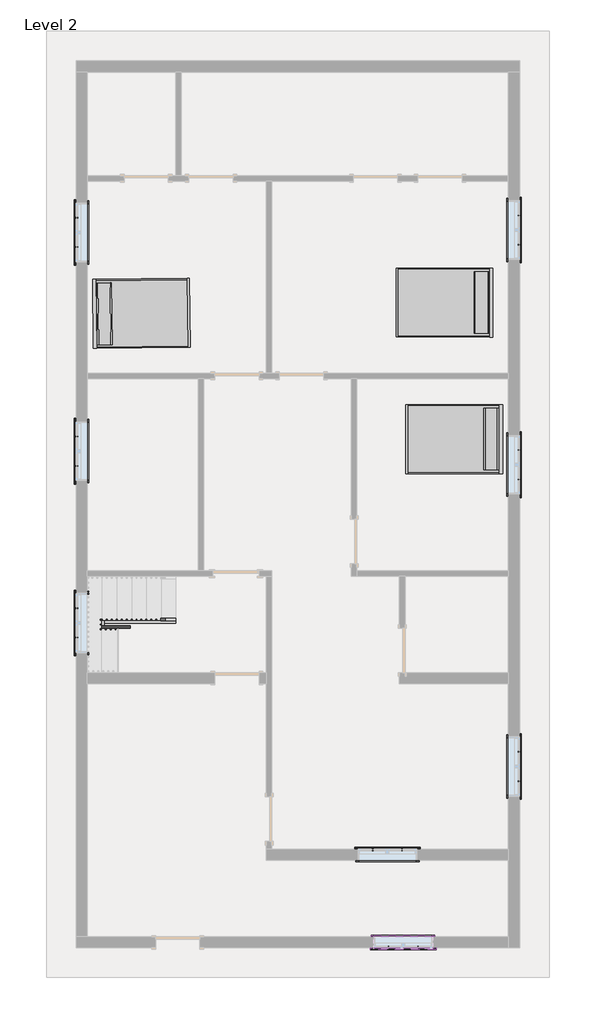
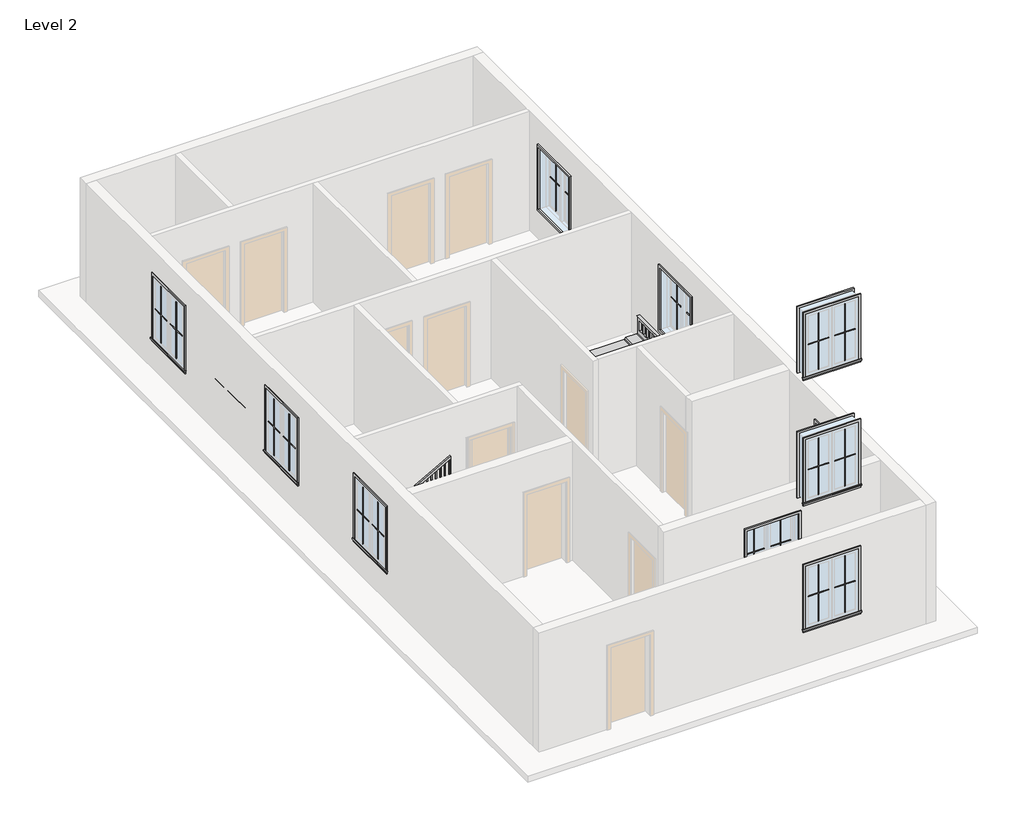
# One storey, part 2 of 2: 40 proxies, 3 furniture elements, 3 members, 1 railing.
"""IFC4 building model written with IfcOpenShell, lengths in millimetres."""

from ifc_helpers import new_model, si_unit, frame, origin, place, context, project, spatial, polyline, outline, extrude, faceted_brep, transform, mapped, element, save
from components import muntin_pattern_2x2_muntin_pattern_2x2_6dad3731, muntin_pattern_2x2_muntin_pattern_2x2_a30a3345, trim_window_exterior_flat_with_sill_92b9b949, trim_window_interior_flat_picture_frame_3bb882cf, furniture_121fd3aa

model = new_model("IFC4")

# Units and contexts
model_context = context("Model", 3, world=origin())
ifc_project = project(units=[si_unit("LENGTHUNIT", "METRE", prefix="MILLI")], contexts=[model_context])

# Site, building, storey
site = spatial("IfcSite", under=ifc_project)
building = spatial("IfcBuilding", under=site)
storey = spatial("IfcBuildingStorey", under=building, Name="Level 2", Elevation=3048.0)

# Proxies
placement = place(None, origin())
muntin_pattern_2x2_muntin_pattern_2x2_shape = muntin_pattern_2x2_muntin_pattern_2x2_6dad3731(model_context)
element("IfcBuildingElementProxy", 1, Name="Muntin Pattern_2x2 : Muntin Pattern_2x2", ObjectType="Muntin Pattern_2x2 : Muntin Pattern_2x2", at=placement, inside=storey, context=model_context, shape_type="MappedRepresentation", body=[
    mapped(muntin_pattern_2x2_muntin_pattern_2x2_shape, transform((1279.525, 5621.3375, 4032.25), x_axis=(0.0, 1.0, 0.0), y_axis=(-1.0, 0.0, 0.0), z_axis=(0.0, 0.0, 1.0))),
])
element("IfcBuildingElementProxy", 2, Name="Muntin Pattern_2x2 : Muntin Pattern_2x2", ObjectType="Muntin Pattern_2x2 : Muntin Pattern_2x2", at=placement, inside=storey, context=model_context, shape_type="MappedRepresentation", body=[
    mapped(muntin_pattern_2x2_muntin_pattern_2x2_shape, transform((1279.525, 10129.8375, 4032.25), x_axis=(0.0, 1.0, 0.0), y_axis=(-1.0, 0.0, 0.0), z_axis=(0.0, 0.0, 1.0))),
])
element("IfcBuildingElementProxy", 3, Name="Muntin Pattern_2x2 : Muntin Pattern_2x2", ObjectType="Muntin Pattern_2x2 : Muntin Pattern_2x2", at=placement, inside=storey, context=model_context, shape_type="MappedRepresentation", body=[
    mapped(muntin_pattern_2x2_muntin_pattern_2x2_shape, transform((10404.475, 10787.0625, 4032.25), x_axis=(0.0, -1.0, 0.0), y_axis=(1.0, 0.0, 0.0), z_axis=(0.0, 0.0, 1.0))),
])
element("IfcBuildingElementProxy", 4, Name="Muntin Pattern_2x2 : Muntin Pattern_2x2", ObjectType="Muntin Pattern_2x2 : Muntin Pattern_2x2", at=placement, inside=storey, context=model_context, shape_type="MappedRepresentation", body=[
    mapped(muntin_pattern_2x2_muntin_pattern_2x2_shape, transform((10404.475, 5948.3625, 4032.25), x_axis=(0.0, -1.0, 0.0), y_axis=(1.0, 0.0, 0.0), z_axis=(0.0, 0.0, 1.0))),
])
element("IfcBuildingElementProxy", 5, Name="Muntin Pattern_2x2 : Muntin Pattern_2x2", ObjectType="Muntin Pattern_2x2 : Muntin Pattern_2x2", at=placement, inside=storey, context=model_context, shape_type="MappedRepresentation", body=[
    mapped(muntin_pattern_2x2_muntin_pattern_2x2_shape, transform((10404.475, -274.6375, 4032.25), x_axis=(0.0, -1.0, 0.0), y_axis=(1.0, 0.0, 0.0), z_axis=(0.0, 0.0, 1.0))),
])
element("IfcBuildingElementProxy", 6, Name="Muntin Pattern_2x2 : Muntin Pattern_2x2", ObjectType="Muntin Pattern_2x2 : Muntin Pattern_2x2", at=placement, inside=storey, context=model_context, shape_type="MappedRepresentation", body=[
    mapped(muntin_pattern_2x2_muntin_pattern_2x2_shape, transform((7386.6375, -2295.525, 4032.25), x_axis=(1.0, 0.0, 0.0), y_axis=(0.0, 1.0, 0.0), z_axis=(0.0, 0.0, 1.0))),
])
element("IfcBuildingElementProxy", 7, Name="Muntin Pattern_2x2 : Muntin Pattern_2x2", ObjectType="Muntin Pattern_2x2 : Muntin Pattern_2x2", at=placement, inside=storey, context=model_context, shape_type="MappedRepresentation", body=[
    mapped(muntin_pattern_2x2_muntin_pattern_2x2_shape, transform((1279.525, 2078.0375, 4032.25), x_axis=(0.0, 1.0, 0.0), y_axis=(-1.0, 0.0, 0.0), z_axis=(0.0, 0.0, 1.0))),
])
element("IfcBuildingElementProxy", 8, Name="Muntin Pattern_2x2 : Muntin Pattern_2x2", ObjectType="Muntin Pattern_2x2 : Muntin Pattern_2x2", at=placement, inside=storey, context=model_context, shape_type="MappedRepresentation", body=[
    mapped(muntin_pattern_2x2_muntin_pattern_2x2_shape, transform((8316.9125, -4308.475, 4140.5050717), x_axis=(-1.0, 0.0, 0.0), y_axis=(0.0, -1.0, 0.0), z_axis=(0.0, 0.0, 1.0))),
])
element("IfcBuildingElementProxy", 9, Name="Muntin Pattern_2x2 : Muntin Pattern_2x2", ObjectType="Muntin Pattern_2x2 : Muntin Pattern_2x2", at=placement, inside=storey, context=model_context, shape_type="MappedRepresentation", body=[
    mapped(muntin_pattern_2x2_muntin_pattern_2x2_shape, transform((8316.9125, -4308.475, 7225.5809921), x_axis=(-1.0, 0.0, 0.0), y_axis=(0.0, -1.0, 0.0), z_axis=(0.0, 0.0, 1.0))),
])
element("IfcBuildingElementProxy", 10, Name="Muntin Pattern_2x2 : Muntin Pattern_2x2", ObjectType="Muntin Pattern_2x2 : Muntin Pattern_2x2", at=placement, inside=storey, context=model_context, shape_type="MappedRepresentation", body=[
    mapped(muntin_pattern_2x2_muntin_pattern_2x2_shape, transform((8316.9125, -4308.475, 10275.7984942), x_axis=(-1.0, 0.0, 0.0), y_axis=(0.0, -1.0, 0.0), z_axis=(0.0, 0.0, 1.0))),
])
muntin_pattern_2x2_muntin_pattern_2x2_2_shape = muntin_pattern_2x2_muntin_pattern_2x2_a30a3345(model_context)
element("IfcBuildingElementProxy", 11, Name="Muntin Pattern_2x2 : Muntin Pattern_2x2", ObjectType="Muntin Pattern_2x2 : Muntin Pattern_2x2", at=placement, inside=storey, context=model_context, shape_type="MappedRepresentation", body=[
    mapped(muntin_pattern_2x2_muntin_pattern_2x2_2_shape, transform((1279.525, 6227.7625, 4032.25), x_axis=(0.0, -1.0, 0.0), y_axis=(1.0, 0.0, 0.0), z_axis=(0.0, 0.0, 1.0))),
])
element("IfcBuildingElementProxy", 12, Name="Muntin Pattern_2x2 : Muntin Pattern_2x2", ObjectType="Muntin Pattern_2x2 : Muntin Pattern_2x2", at=placement, inside=storey, context=model_context, shape_type="MappedRepresentation", body=[
    mapped(muntin_pattern_2x2_muntin_pattern_2x2_2_shape, transform((1279.525, 10736.2625, 4032.25), x_axis=(0.0, -1.0, 0.0), y_axis=(1.0, 0.0, 0.0), z_axis=(0.0, 0.0, 1.0))),
])
element("IfcBuildingElementProxy", 13, Name="Muntin Pattern_2x2 : Muntin Pattern_2x2", ObjectType="Muntin Pattern_2x2 : Muntin Pattern_2x2", at=placement, inside=storey, context=model_context, shape_type="MappedRepresentation", body=[
    mapped(muntin_pattern_2x2_muntin_pattern_2x2_2_shape, transform((10404.475, 10180.6375, 4032.25), x_axis=(0.0, 1.0, 0.0), y_axis=(-1.0, 0.0, 0.0), z_axis=(0.0, 0.0, 1.0))),
])
element("IfcBuildingElementProxy", 14, Name="Muntin Pattern_2x2 : Muntin Pattern_2x2", ObjectType="Muntin Pattern_2x2 : Muntin Pattern_2x2", at=placement, inside=storey, context=model_context, shape_type="MappedRepresentation", body=[
    mapped(muntin_pattern_2x2_muntin_pattern_2x2_2_shape, transform((10404.475, 5341.9375, 4032.25), x_axis=(0.0, 1.0, 0.0), y_axis=(-1.0, 0.0, 0.0), z_axis=(0.0, 0.0, 1.0))),
])
element("IfcBuildingElementProxy", 15, Name="Muntin Pattern_2x2 : Muntin Pattern_2x2", ObjectType="Muntin Pattern_2x2 : Muntin Pattern_2x2", at=placement, inside=storey, context=model_context, shape_type="MappedRepresentation", body=[
    mapped(muntin_pattern_2x2_muntin_pattern_2x2_2_shape, transform((10404.475, -881.0625, 4032.25), x_axis=(0.0, 1.0, 0.0), y_axis=(-1.0, 0.0, 0.0), z_axis=(0.0, 0.0, 1.0))),
])
element("IfcBuildingElementProxy", 16, Name="Muntin Pattern_2x2 : Muntin Pattern_2x2", ObjectType="Muntin Pattern_2x2 : Muntin Pattern_2x2", at=placement, inside=storey, context=model_context, shape_type="MappedRepresentation", body=[
    mapped(muntin_pattern_2x2_muntin_pattern_2x2_2_shape, transform((7993.0625, -2295.525, 4032.25), x_axis=(-1.0, 0.0, 0.0), y_axis=(0.0, -1.0, 0.0), z_axis=(0.0, 0.0, 1.0))),
])
element("IfcBuildingElementProxy", 17, Name="Muntin Pattern_2x2 : Muntin Pattern_2x2", ObjectType="Muntin Pattern_2x2 : Muntin Pattern_2x2", at=placement, inside=storey, context=model_context, shape_type="MappedRepresentation", body=[
    mapped(muntin_pattern_2x2_muntin_pattern_2x2_2_shape, transform((1279.525, 2684.4625, 4032.25), x_axis=(0.0, -1.0, 0.0), y_axis=(1.0, 0.0, 0.0), z_axis=(0.0, 0.0, 1.0))),
])
element("IfcBuildingElementProxy", 18, Name="Muntin Pattern_2x2 : Muntin Pattern_2x2", ObjectType="Muntin Pattern_2x2 : Muntin Pattern_2x2", at=placement, inside=storey, context=model_context, shape_type="MappedRepresentation", body=[
    mapped(muntin_pattern_2x2_muntin_pattern_2x2_2_shape, transform((7710.4875, -4308.475, 4140.5050717), x_axis=(1.0, 0.0, 0.0), y_axis=(0.0, 1.0, 0.0), z_axis=(0.0, 0.0, 1.0))),
])
element("IfcBuildingElementProxy", 19, Name="Muntin Pattern_2x2 : Muntin Pattern_2x2", ObjectType="Muntin Pattern_2x2 : Muntin Pattern_2x2", at=placement, inside=storey, context=model_context, shape_type="MappedRepresentation", body=[
    mapped(muntin_pattern_2x2_muntin_pattern_2x2_2_shape, transform((7710.4875, -4308.475, 7225.5809921), x_axis=(1.0, 0.0, 0.0), y_axis=(0.0, 1.0, 0.0), z_axis=(0.0, 0.0, 1.0))),
])
element("IfcBuildingElementProxy", 20, Name="Muntin Pattern_2x2 : Muntin Pattern_2x2", ObjectType="Muntin Pattern_2x2 : Muntin Pattern_2x2", at=placement, inside=storey, context=model_context, shape_type="MappedRepresentation", body=[
    mapped(muntin_pattern_2x2_muntin_pattern_2x2_2_shape, transform((7710.4875, -4308.475, 10275.7984942), x_axis=(1.0, 0.0, 0.0), y_axis=(0.0, 1.0, 0.0), z_axis=(0.0, 0.0, 1.0))),
])
trim_window_exterior_flat_with_sill_shape = trim_window_exterior_flat_with_sill_92b9b949(model_context)
element("IfcBuildingElementProxy", 21, Name="Trim-Window-Exterior-Flat : with Sill", ObjectType="Trim-Window-Exterior-Flat : with Sill", at=placement, inside=storey, context=model_context, shape_type="MappedRepresentation", body=[
    mapped(trim_window_exterior_flat_with_sill_shape, transform((1270.0, 5924.55, 5486.4), x_axis=(0.0, -1.0, 0.0), y_axis=(0.0, 0.0, 1.0), z_axis=(-1.0, 0.0, 0.0))),
])
element("IfcBuildingElementProxy", 22, Name="Trim-Window-Exterior-Flat : with Sill", ObjectType="Trim-Window-Exterior-Flat : with Sill", at=placement, inside=storey, context=model_context, shape_type="MappedRepresentation", body=[
    mapped(trim_window_exterior_flat_with_sill_shape, transform((1270.0, 10433.05, 5486.4), x_axis=(0.0, -1.0, 0.0), y_axis=(0.0, 0.0, 1.0), z_axis=(-1.0, 0.0, 0.0))),
])
element("IfcBuildingElementProxy", 23, Name="Trim-Window-Exterior-Flat : with Sill", ObjectType="Trim-Window-Exterior-Flat : with Sill", at=placement, inside=storey, context=model_context, shape_type="MappedRepresentation", body=[
    mapped(trim_window_exterior_flat_with_sill_shape, transform((10414.0, 10483.85, 5486.4), x_axis=(0.0, 1.0, 0.0), y_axis=(0.0, 0.0, 1.0), z_axis=(1.0, 0.0, 0.0))),
])
element("IfcBuildingElementProxy", 24, Name="Trim-Window-Exterior-Flat : with Sill", ObjectType="Trim-Window-Exterior-Flat : with Sill", at=placement, inside=storey, context=model_context, shape_type="MappedRepresentation", body=[
    mapped(trim_window_exterior_flat_with_sill_shape, transform((10414.0, 5645.15, 5486.4), x_axis=(0.0, 1.0, 0.0), y_axis=(0.0, 0.0, 1.0), z_axis=(1.0, 0.0, 0.0))),
])
element("IfcBuildingElementProxy", 25, Name="Trim-Window-Exterior-Flat : with Sill", ObjectType="Trim-Window-Exterior-Flat : with Sill", at=placement, inside=storey, context=model_context, shape_type="MappedRepresentation", body=[
    mapped(trim_window_exterior_flat_with_sill_shape, transform((10414.0, -577.85, 5486.4), x_axis=(0.0, 1.0, 0.0), y_axis=(0.0, 0.0, 1.0), z_axis=(1.0, 0.0, 0.0))),
])
element("IfcBuildingElementProxy", 26, Name="Trim-Window-Exterior-Flat : with Sill", ObjectType="Trim-Window-Exterior-Flat : with Sill", at=placement, inside=storey, context=model_context, shape_type="MappedRepresentation", body=[
    mapped(trim_window_exterior_flat_with_sill_shape, transform((7689.85, -2286.0, 5486.4), x_axis=(-1.0, 0.0, 0.0), y_axis=(0.0, 0.0, 1.0), z_axis=(0.0, 1.0, 0.0))),
])
element("IfcBuildingElementProxy", 27, Name="Trim-Window-Exterior-Flat : with Sill", ObjectType="Trim-Window-Exterior-Flat : with Sill", at=placement, inside=storey, context=model_context, shape_type="MappedRepresentation", body=[
    mapped(trim_window_exterior_flat_with_sill_shape, transform((1270.0, 2381.25, 5486.4), x_axis=(0.0, -1.0, 0.0), y_axis=(0.0, 0.0, 1.0), z_axis=(-1.0, 0.0, 0.0))),
])
element("IfcBuildingElementProxy", 28, Name="Trim-Window-Exterior-Flat : with Sill", ObjectType="Trim-Window-Exterior-Flat : with Sill", at=placement, inside=storey, context=model_context, shape_type="MappedRepresentation", body=[
    mapped(trim_window_exterior_flat_with_sill_shape, transform((8013.7, -4318.0, 5594.6550717), x_axis=(1.0, 0.0, 0.0), y_axis=(0.0, 0.0, 1.0), z_axis=(0.0, -1.0, 0.0))),
])
element("IfcBuildingElementProxy", 29, Name="Trim-Window-Exterior-Flat : with Sill", ObjectType="Trim-Window-Exterior-Flat : with Sill", at=placement, inside=storey, context=model_context, shape_type="MappedRepresentation", body=[
    mapped(trim_window_exterior_flat_with_sill_shape, transform((8013.7, -4318.0, 8679.7309921), x_axis=(1.0, 0.0, 0.0), y_axis=(0.0, 0.0, 1.0), z_axis=(0.0, -1.0, 0.0))),
])
element("IfcBuildingElementProxy", 30, Name="Trim-Window-Exterior-Flat : with Sill", ObjectType="Trim-Window-Exterior-Flat : with Sill", at=placement, inside=storey, context=model_context, shape_type="MappedRepresentation", body=[
    mapped(trim_window_exterior_flat_with_sill_shape, transform((8013.7, -4318.0, 11729.9484942), x_axis=(1.0, 0.0, 0.0), y_axis=(0.0, 0.0, 1.0), z_axis=(0.0, -1.0, 0.0))),
])
trim_window_interior_flat_picture_frame_shape = trim_window_interior_flat_picture_frame_3bb882cf(model_context)
element("IfcBuildingElementProxy", 31, Name="Trim-Window-Interior-Flat : Picture Frame", ObjectType="Trim-Window-Interior-Flat : Picture Frame", at=placement, inside=storey, context=model_context, shape_type="MappedRepresentation", body=[
    mapped(trim_window_interior_flat_picture_frame_shape, transform((1498.6, 5924.55, 5486.4), x_axis=(0.0, 1.0, 0.0), y_axis=(0.0, 0.0, 1.0), z_axis=(1.0, 0.0, 0.0))),
])
element("IfcBuildingElementProxy", 32, Name="Trim-Window-Interior-Flat : Picture Frame", ObjectType="Trim-Window-Interior-Flat : Picture Frame", at=placement, inside=storey, context=model_context, shape_type="MappedRepresentation", body=[
    mapped(trim_window_interior_flat_picture_frame_shape, transform((1498.6, 10433.05, 5486.4), x_axis=(0.0, 1.0, 0.0), y_axis=(0.0, 0.0, 1.0), z_axis=(1.0, 0.0, 0.0))),
])
element("IfcBuildingElementProxy", 33, Name="Trim-Window-Interior-Flat : Picture Frame", ObjectType="Trim-Window-Interior-Flat : Picture Frame", at=placement, inside=storey, context=model_context, shape_type="MappedRepresentation", body=[
    mapped(trim_window_interior_flat_picture_frame_shape, transform((10185.4, 10483.85, 5486.4), x_axis=(0.0, -1.0, 0.0), y_axis=(0.0, 0.0, 1.0), z_axis=(-1.0, 0.0, 0.0))),
])
element("IfcBuildingElementProxy", 34, Name="Trim-Window-Interior-Flat : Picture Frame", ObjectType="Trim-Window-Interior-Flat : Picture Frame", at=placement, inside=storey, context=model_context, shape_type="MappedRepresentation", body=[
    mapped(trim_window_interior_flat_picture_frame_shape, transform((10185.4, 5645.15, 5486.4), x_axis=(0.0, -1.0, 0.0), y_axis=(0.0, 0.0, 1.0), z_axis=(-1.0, 0.0, 0.0))),
])
element("IfcBuildingElementProxy", 35, Name="Trim-Window-Interior-Flat : Picture Frame", ObjectType="Trim-Window-Interior-Flat : Picture Frame", at=placement, inside=storey, context=model_context, shape_type="MappedRepresentation", body=[
    mapped(trim_window_interior_flat_picture_frame_shape, transform((10185.4, -577.85, 5486.4), x_axis=(0.0, -1.0, 0.0), y_axis=(0.0, 0.0, 1.0), z_axis=(-1.0, 0.0, 0.0))),
])
element("IfcBuildingElementProxy", 36, Name="Trim-Window-Interior-Flat : Picture Frame", ObjectType="Trim-Window-Interior-Flat : Picture Frame", at=placement, inside=storey, context=model_context, shape_type="MappedRepresentation", body=[
    mapped(trim_window_interior_flat_picture_frame_shape, transform((7689.85, -2514.6, 5486.4), x_axis=(1.0, 0.0, 0.0), y_axis=(0.0, 0.0, 1.0), z_axis=(0.0, -1.0, 0.0))),
])
element("IfcBuildingElementProxy", 37, Name="Trim-Window-Interior-Flat : Picture Frame", ObjectType="Trim-Window-Interior-Flat : Picture Frame", at=placement, inside=storey, context=model_context, shape_type="MappedRepresentation", body=[
    mapped(trim_window_interior_flat_picture_frame_shape, transform((1498.6, 2381.25, 5486.4), x_axis=(0.0, 1.0, 0.0), y_axis=(0.0, 0.0, 1.0), z_axis=(1.0, 0.0, 0.0))),
])
element("IfcBuildingElementProxy", 38, Name="Trim-Window-Interior-Flat : Picture Frame", ObjectType="Trim-Window-Interior-Flat : Picture Frame", at=placement, inside=storey, context=model_context, shape_type="MappedRepresentation", body=[
    mapped(trim_window_interior_flat_picture_frame_shape, transform((8013.7, -4089.4, 5594.6550717), x_axis=(-1.0, 0.0, 0.0), y_axis=(0.0, 0.0, 1.0), z_axis=(0.0, 1.0, 0.0))),
])
element("IfcBuildingElementProxy", 39, Name="Trim-Window-Interior-Flat : Picture Frame", ObjectType="Trim-Window-Interior-Flat : Picture Frame", at=placement, inside=storey, context=model_context, shape_type="MappedRepresentation", body=[
    mapped(trim_window_interior_flat_picture_frame_shape, transform((8013.7, -4089.4, 8679.7309921), x_axis=(-1.0, 0.0, 0.0), y_axis=(0.0, 0.0, 1.0), z_axis=(0.0, 1.0, 0.0))),
])
element("IfcBuildingElementProxy", 40, Name="Trim-Window-Interior-Flat : Picture Frame", ObjectType="Trim-Window-Interior-Flat : Picture Frame", at=placement, inside=storey, context=model_context, shape_type="MappedRepresentation", body=[
    mapped(trim_window_interior_flat_picture_frame_shape, transform((8013.7, -4089.4, 11729.9484942), x_axis=(-1.0, 0.0, 0.0), y_axis=(0.0, 0.0, 1.0), z_axis=(0.0, 1.0, 0.0))),
])

# Furniture
furniture_shape = furniture_121fd3aa(model_context)
element("IfcFurniture", 41, ObjectType="Bed-Shaker : Double 56\" x 78\"", at=placement, inside=storey, context=model_context, shape_type="MappedRepresentation", body=[
    mapped(furniture_shape, transform((9849.8308516, 8970.3536289, 3048.0), x_axis=(0.0, -1.0, 0.0), y_axis=(1.0, 0.0, 0.0), z_axis=(0.0, 0.0, 1.0))),
])
element("IfcFurniture", 42, ObjectType="Bed-Shaker : Double 56\" x 78\"", at=placement, inside=storey, context=model_context, shape_type="MappedRepresentation", body=[
    mapped(furniture_shape, transform((10050.5002502, 6155.12029, 3048.0), x_axis=(0.0, -1.0, 0.0), y_axis=(1.0, 0.0, 0.0), z_axis=(0.0, 0.0, 1.0))),
])
element("IfcFurniture", 43, ObjectType="Bed-Shaker : Double 56\" x 78\"", at=placement, inside=storey, context=model_context, shape_type="MappedRepresentation", body=[
    mapped(furniture_shape, transform((1630.8006063, 8772.9712322, 3048.0), x_axis=(-0.01124472055544287, 0.9999367761311863, 0.0), y_axis=(-0.9999367761311863, -0.01124472055544287, 0.0), z_axis=(0.0, 0.0, 1.0))),
])

# Members
element("IfcMember", 44, ObjectType="Stringer - 2\" Width", at=placement, inside=storey, context=model_context, shape_type="SweptSolid", body=[
    extrude(outline(polyline([(3048.0, 3327.4), (3255.5983948, 3327.4), (4074.0428392, 1854.2), (3725.3641651, 1854.2), (3048.0, 3073.4554972), (3048.0, 3327.4)])), frame((0.0, 2374.9, 0.0), z_axis=(0.0, 1.0, 0.0), x_axis=(0.0, 0.0, 1.0)), (0.0, 0.0, 1.0), 50.8),
])
element("IfcMember", 45, ObjectType="Stringer - 2\" Width", at=placement, inside=storey, context=model_context, shape_type="SweptSolid", body=[
    extrude(outline(polyline([(1803.4, 2425.7), (1854.2, 2425.7), (1854.2, 2324.1), (1803.4, 2324.1), (1803.4, 2425.7)])), frame((0.0, 0.0, 3835.4), z_axis=(0.0, 0.0, 1.0), x_axis=(1.0, 0.0, 0.0)), (0.0, 0.0, 1.0), 304.8),
])
element("IfcMember", 46, ObjectType="Stringer - 2\" Width", at=placement, inside=storey, context=model_context, shape_type="SweptSolid", body=[
    extrude(outline(polyline([(4271.5983948, 1803.4), (3922.9197207, 1803.4), (4600.253054, 3022.6), (4948.9317281, 3022.6), (4271.5983948, 1803.4)])), frame((0.0, 2273.3, 0.0), z_axis=(0.0, 1.0, 0.0), x_axis=(0.0, 0.0, 1.0)), (0.0, 0.0, 1.0), 50.8),
])

# Railing
element("IfcRailing", 47, ObjectType="Handrail - Rectangular", at=placement, inside=storey, context=model_context, shape_type="SolidModel", body=[
    faceted_brep([(3327.4, 2425.7, 4131.7333333), (3327.4, 2425.7, 4073.620221), (3327.4, 2476.5, 4073.620221), (3327.4, 2476.5, 4131.7333333), (1879.6, 2425.7, 4936.0666667), (1828.8, 2425.7, 4906.1757765), (1828.8, 2476.5, 4906.1757765), (1879.6, 2476.5, 4936.0666667), (1879.6, 2425.7, 4978.4), (1828.8, 2425.7, 4927.6), (1828.8, 2476.5, 4927.6), (1879.6, 2476.5, 4978.4), (1803.4, 2425.7, 4978.4), (1803.4, 2425.7, 4927.6), (1752.6, 2476.5, 4927.6), (1752.6, 2476.5, 4978.4), (1803.4, 2349.5, 4978.4), (1803.4, 2298.7, 4927.6), (1752.6, 2298.7, 4927.6), (1752.6, 2349.5, 4978.4), (1803.4, 2349.5, 5190.0666667), (1803.4, 2298.7, 5139.2666667), (1752.6, 2298.7, 5139.2666667), (1752.6, 2349.5, 5190.0666667), (1803.4, 2273.3, 5190.0666667), (1803.4, 2273.3, 5139.2666667), (1752.6, 2222.5, 5139.2666667), (1752.6, 2222.5, 5190.0666667), (1879.6, 2273.3, 5190.0666667), (1892.7636022, 2273.3, 5139.2666667), (1892.7636022, 2222.5, 5139.2666667), (1879.6, 2222.5, 5190.0666667), (3022.6, 2273.3, 5825.0666667), (3022.6, 2222.5, 5825.0666667), (3022.6, 2222.5, 5766.9535543), (3022.6, 2273.3, 5766.9535543)], [[[0, 1, 2, 3]], [[1, 0, 4, 5]], [[2, 1, 5, 6]], [[3, 2, 6, 7]], [[0, 3, 7, 4]], [[5, 4, 8, 9]], [[6, 5, 9, 10]], [[7, 6, 10, 11]], [[4, 7, 11, 8]], [[9, 8, 12, 13]], [[10, 9, 13, 14]], [[11, 10, 14, 15]], [[8, 11, 15, 12]], [[13, 12, 16, 17]], [[14, 13, 17, 18]], [[15, 14, 18, 19]], [[12, 15, 19, 16]], [[17, 16, 20, 21]], [[18, 17, 21, 22]], [[19, 18, 22, 23]], [[16, 19, 23, 20]], [[21, 20, 24, 25]], [[22, 21, 25, 26]], [[23, 22, 26, 27]], [[20, 23, 27, 24]], [[25, 24, 28, 29]], [[26, 25, 29, 30]], [[27, 26, 30, 31]], [[24, 27, 31, 28]], [[32, 33, 34, 35]], [[29, 28, 32, 35]], [[30, 29, 35, 34]], [[31, 30, 34, 33]], [[28, 31, 33, 32]]]),
    extrude(outline(polyline([(5747.5507765, 2987.675), (4741.3333333, 2987.675), (4741.3333333, 3006.725), (5758.1341099, 3006.725), (5747.5507765, 2987.675)])), frame((0.0, 2238.375, 0.0), z_axis=(0.0, 1.0, 0.0), x_axis=(0.0, 0.0, 1.0)), (0.0, 0.0, 1.0), 19.05),
    extrude(outline(polyline([(5691.1063321, 2886.075), (4741.3333333, 2886.075), (4741.3333333, 2905.125), (5701.6896654, 2905.125), (5691.1063321, 2886.075)])), frame((0.0, 2238.375, 0.0), z_axis=(0.0, 1.0, 0.0), x_axis=(0.0, 0.0, 1.0)), (0.0, 0.0, 1.0), 19.05),
    extrude(outline(polyline([(5634.6618876, 2784.475), (4741.3333333, 2784.475), (4741.3333333, 2803.525), (5645.245221, 2803.525), (5634.6618876, 2784.475)])), frame((0.0, 2238.375, 0.0), z_axis=(0.0, 1.0, 0.0), x_axis=(0.0, 0.0, 1.0)), (0.0, 0.0, 1.0), 19.05),
    extrude(outline(polyline([(5578.2174432, 2682.875), (4572.0, 2682.875), (4572.0, 2701.925), (5588.8007765, 2701.925), (5578.2174432, 2682.875)])), frame((0.0, 2238.375, 0.0), z_axis=(0.0, 1.0, 0.0), x_axis=(0.0, 0.0, 1.0)), (0.0, 0.0, 1.0), 19.05),
    extrude(outline(polyline([(5521.7729988, 2581.275), (4572.0, 2581.275), (4572.0, 2600.325), (5532.3563321, 2600.325), (5521.7729988, 2581.275)])), frame((0.0, 2238.375, 0.0), z_axis=(0.0, 1.0, 0.0), x_axis=(0.0, 0.0, 1.0)), (0.0, 0.0, 1.0), 19.05),
    extrude(outline(polyline([(5465.3285543, 2479.675), (4572.0, 2479.675), (4572.0, 2498.725), (5475.9118876, 2498.725), (5465.3285543, 2479.675)])), frame((0.0, 2238.375, 0.0), z_axis=(0.0, 1.0, 0.0), x_axis=(0.0, 0.0, 1.0)), (0.0, 0.0, 1.0), 19.05),
    extrude(outline(polyline([(5408.8841099, 2378.075), (4402.6666667, 2378.075), (4402.6666667, 2397.125), (5419.4674432, 2397.125), (5408.8841099, 2378.075)])), frame((0.0, 2238.375, 0.0), z_axis=(0.0, 1.0, 0.0), x_axis=(0.0, 0.0, 1.0)), (0.0, 0.0, 1.0), 19.05),
    extrude(outline(polyline([(5352.4396654, 2276.475), (4402.6666667, 2276.475), (4402.6666667, 2295.525), (5363.0229988, 2295.525), (5352.4396654, 2276.475)])), frame((0.0, 2238.375, 0.0), z_axis=(0.0, 1.0, 0.0), x_axis=(0.0, 0.0, 1.0)), (0.0, 0.0, 1.0), 19.05),
    extrude(outline(polyline([(5295.995221, 2174.875), (4402.6666667, 2174.875), (4402.6666667, 2193.925), (5306.5785543, 2193.925), (5295.995221, 2174.875)])), frame((0.0, 2238.375, 0.0), z_axis=(0.0, 1.0, 0.0), x_axis=(0.0, 0.0, 1.0)), (0.0, 0.0, 1.0), 19.05),
    extrude(outline(polyline([(5239.5507765, 2073.275), (4233.3333333, 2073.275), (4233.3333333, 2092.325), (5250.1341099, 2092.325), (5239.5507765, 2073.275)])), frame((0.0, 2238.375, 0.0), z_axis=(0.0, 1.0, 0.0), x_axis=(0.0, 0.0, 1.0)), (0.0, 0.0, 1.0), 19.05),
    extrude(outline(polyline([(5183.1063321, 1971.675), (4233.3333333, 1971.675), (4233.3333333, 1990.725), (5193.6896654, 1990.725), (5183.1063321, 1971.675)])), frame((0.0, 2238.375, 0.0), z_axis=(0.0, 1.0, 0.0), x_axis=(0.0, 0.0, 1.0)), (0.0, 0.0, 1.0), 19.05),
    extrude(outline(polyline([(5126.6618876, 1870.075), (4233.3333333, 1870.075), (4233.3333333, 1889.125), (5137.245221, 1889.125), (5126.6618876, 1870.075)])), frame((0.0, 2238.375, 0.0), z_axis=(0.0, 1.0, 0.0), x_axis=(0.0, 0.0, 1.0)), (0.0, 0.0, 1.0), 19.05),
    extrude(outline(polyline([(1787.525, 2359.025), (1787.525, 2339.975), (1768.475, 2339.975), (1768.475, 2359.025), (1787.525, 2359.025)])), frame((0.0, 0.0, 4064.0), z_axis=(0.0, 0.0, 1.0), x_axis=(1.0, 0.0, 0.0)), (0.0, 0.0, 1.0), 863.6),
    extrude(outline(polyline([(1812.925, 2441.575), (1793.875, 2441.575), (1793.875, 2460.625), (1812.925, 2460.625), (1812.925, 2441.575)])), frame((0.0, 0.0, 4064.0), z_axis=(0.0, 0.0, 1.0), x_axis=(1.0, 0.0, 0.0)), (0.0, 0.0, 1.0), 863.6),
    extrude(outline(polyline([(4869.1341099, 1895.475), (3894.6666667, 1895.475), (3894.6666667, 1914.525), (4858.5507765, 1914.525), (4869.1341099, 1895.475)])), frame((0.0, 2441.575, 0.0), z_axis=(0.0, 1.0, 0.0), x_axis=(0.0, 0.0, 1.0)), (0.0, 0.0, 1.0), 19.05),
    extrude(outline(polyline([(4812.6896654, 1997.075), (3894.6666667, 1997.075), (3894.6666667, 2016.125), (4802.1063321, 2016.125), (4812.6896654, 1997.075)])), frame((0.0, 2441.575, 0.0), z_axis=(0.0, 1.0, 0.0), x_axis=(0.0, 0.0, 1.0)), (0.0, 0.0, 1.0), 19.05),
    extrude(outline(polyline([(4756.245221, 2098.675), (3894.6666667, 2098.675), (3894.6666667, 2117.725), (4745.6618876, 2117.725), (4756.245221, 2098.675)])), frame((0.0, 2441.575, 0.0), z_axis=(0.0, 1.0, 0.0), x_axis=(0.0, 0.0, 1.0)), (0.0, 0.0, 1.0), 19.05),
    extrude(outline(polyline([(4699.8007765, 2200.275), (3725.3333333, 2200.275), (3725.3333333, 2219.325), (4689.2174432, 2219.325), (4699.8007765, 2200.275)])), frame((0.0, 2441.575, 0.0), z_axis=(0.0, 1.0, 0.0), x_axis=(0.0, 0.0, 1.0)), (0.0, 0.0, 1.0), 19.05),
    extrude(outline(polyline([(4643.3563321, 2301.875), (3725.3333333, 2301.875), (3725.3333333, 2320.925), (4632.7729988, 2320.925), (4643.3563321, 2301.875)])), frame((0.0, 2441.575, 0.0), z_axis=(0.0, 1.0, 0.0), x_axis=(0.0, 0.0, 1.0)), (0.0, 0.0, 1.0), 19.05),
    extrude(outline(polyline([(4586.9118876, 2403.475), (3725.3333333, 2403.475), (3725.3333333, 2422.525), (4576.3285543, 2422.525), (4586.9118876, 2403.475)])), frame((0.0, 2441.575, 0.0), z_axis=(0.0, 1.0, 0.0), x_axis=(0.0, 0.0, 1.0)), (0.0, 0.0, 1.0), 19.05),
    extrude(outline(polyline([(4530.4674432, 2505.075), (3556.0, 2505.075), (3556.0, 2524.125), (4519.8841099, 2524.125), (4530.4674432, 2505.075)])), frame((0.0, 2441.575, 0.0), z_axis=(0.0, 1.0, 0.0), x_axis=(0.0, 0.0, 1.0)), (0.0, 0.0, 1.0), 19.05),
    extrude(outline(polyline([(4474.0229988, 2606.675), (3556.0, 2606.675), (3556.0, 2625.725), (4463.4396654, 2625.725), (4474.0229988, 2606.675)])), frame((0.0, 2441.575, 0.0), z_axis=(0.0, 1.0, 0.0), x_axis=(0.0, 0.0, 1.0)), (0.0, 0.0, 1.0), 19.05),
    extrude(outline(polyline([(4417.5785543, 2708.275), (3556.0, 2708.275), (3556.0, 2727.325), (4406.995221, 2727.325), (4417.5785543, 2708.275)])), frame((0.0, 2441.575, 0.0), z_axis=(0.0, 1.0, 0.0), x_axis=(0.0, 0.0, 1.0)), (0.0, 0.0, 1.0), 19.05),
    extrude(outline(polyline([(4361.1341099, 2809.875), (3386.6666667, 2809.875), (3386.6666667, 2828.925), (4350.5507765, 2828.925), (4361.1341099, 2809.875)])), frame((0.0, 2441.575, 0.0), z_axis=(0.0, 1.0, 0.0), x_axis=(0.0, 0.0, 1.0)), (0.0, 0.0, 1.0), 19.05),
    extrude(outline(polyline([(4304.6896654, 2911.475), (3386.6666667, 2911.475), (3386.6666667, 2930.525), (4294.1063321, 2930.525), (4304.6896654, 2911.475)])), frame((0.0, 2441.575, 0.0), z_axis=(0.0, 1.0, 0.0), x_axis=(0.0, 0.0, 1.0)), (0.0, 0.0, 1.0), 19.05),
    extrude(outline(polyline([(4248.245221, 3013.075), (3386.6666667, 3013.075), (3386.6666667, 3032.125), (4237.6618876, 3032.125), (4248.245221, 3013.075)])), frame((0.0, 2441.575, 0.0), z_axis=(0.0, 1.0, 0.0), x_axis=(0.0, 0.0, 1.0)), (0.0, 0.0, 1.0), 19.05),
    extrude(outline(polyline([(4191.8007765, 3114.675), (3217.3333333, 3114.675), (3217.3333333, 3133.725), (4181.2174432, 3133.725), (4191.8007765, 3114.675)])), frame((0.0, 2441.575, 0.0), z_axis=(0.0, 1.0, 0.0), x_axis=(0.0, 0.0, 1.0)), (0.0, 0.0, 1.0), 19.05),
    extrude(outline(polyline([(4135.3563321, 3216.275), (3217.3333333, 3216.275), (3217.3333333, 3235.325), (4124.7729988, 3235.325), (4135.3563321, 3216.275)])), frame((0.0, 2441.575, 0.0), z_axis=(0.0, 1.0, 0.0), x_axis=(0.0, 0.0, 1.0)), (0.0, 0.0, 1.0), 19.05),
    extrude(outline(polyline([(1787.525, 2257.425), (1787.525, 2238.375), (1768.475, 2238.375), (1768.475, 2257.425), (1787.525, 2257.425)])), frame((0.0, 0.0, 4064.0), z_axis=(0.0, 0.0, 1.0), x_axis=(1.0, 0.0, 0.0)), (0.0, 0.0, 1.0), 1075.2666667),
    extrude(outline(polyline([(1787.525, 2441.575), (1768.475, 2441.575), (1768.475, 2460.625), (1787.525, 2460.625), (1787.525, 2441.575)])), frame((0.0, 0.0, 4064.0), z_axis=(0.0, 0.0, 1.0), x_axis=(1.0, 0.0, 0.0)), (0.0, 0.0, 1.0), 863.6),
    extrude(outline(polyline([(5756.370221, 3003.55), (4741.3333333, 3003.55), (4741.3333333, 3022.6), (5766.9535543, 3022.6), (5756.370221, 3003.55)])), frame((0.0, 2238.375, 0.0), z_axis=(0.0, 1.0, 0.0), x_axis=(0.0, 0.0, 1.0)), (0.0, 0.0, 1.0), 19.05),
    extrude(outline(polyline([(4084.2035543, 3308.35), (3217.3333333, 3308.35), (3217.3333333, 3327.4), (4073.620221, 3327.4), (4084.2035543, 3308.35)])), frame((0.0, 2441.575, 0.0), z_axis=(0.0, 1.0, 0.0), x_axis=(0.0, 0.0, 1.0)), (0.0, 0.0, 1.0), 19.05),
])

save(model, "model.ifc")

# Revit data of these elements
# Type "Muntin Pattern_2x2 : Muntin Pattern_2x2"
#   Width [instance default] = 4' - 0"
#   Thickness = 0' - 0 1/2"
#   Height [instance default] = 4' - 0"
#   Distance = 0' - 0 3/4"
#   Interior Material [instance default] = none
#   Exterior Material [instance default] = none
#   Default Elevation = 0
# Type "Trim-Window-Exterior-Flat : with Sill"
#   Trim Width = 0' - 2 1/4"
#   Trim Thickness_Picture Frame = 0' - 1 1/4"
#   Trim Thickness_with Sill = 0' - 0 3/4"
#   Sill Thickness = 0' - 1 1/4"
#   Opening Width [instance default] = 2' - 0"
#   Opening Height [instance default] = 3' - 0"
#   Default Elevation = 4' - 0"
#   Sill = yes
#   Picture Frame = no
#   Trim Material [instance default] = none
# Type "Trim-Window-Interior-Flat : Picture Frame"
#   Trim Thickness_Picture Frame = 0' - 1 1/4"
#   Trim Width = 0' - 2 1/4"
#   Trim Thickness_with Sill = 0' - 0 3/4"
#   Sill Thickness = 0' - 1 1/4"
#   Opening Width [instance default] = 2' - 0"
#   Opening Height [instance default] = 3' - 0"
#   Default Elevation = 4' - 0"
#   Sill = no
#   Picture Frame = yes
#   Trim Material [instance default] = none
# Type "Bed-Shaker : Double 56\" x 78\""
#   Assembly Code = "E2020200"
#   Length = 6' - 6"
#   Width = 4' - 8"
#   Frame Material = Birch
#   Mattress Material = Linen, White
#   Default Elevation = 0
# Type "Handrail - Rectangular"
#   Assembly Code = "C2010400"
#   built-in parameter 1008612 = 0.0416667 (stored number, unit not read)
#   built-in parameter 1008611 = 0.0416667 (stored number, unit not read)
#   built-in parameter 1008609 = 0.333333 (stored number, unit not read)
#   built-in parameter 1008604 = 0.166667 (stored number, unit not read)
#   built-in parameter 1008603 = 0.166667 (stored number, unit not read)
#   Railing Height = 3' - 0"
#   built-in parameter 1008630 = 2
#   built-in parameter 1008610 = 2
#   built-in parameter 1008618 = Baluster - Square : 3/4"
# Elements 1, 2, 3, 4, 5, 6, 7, 8, 9, 10, 11, 12, 13, 14, 15, 16, 17, 18, 19, 20 (IfcBuildingElementProxy, "Muntin Pattern_2x2 : Muntin Pattern_2x2")
#   Width = 1' - 6 5/8"
#   Height = 4' - 6 1/2"
#   Interior Material = Wood - Stained
#   Exterior Material = Clad - White
#   Phase Created = New Construction
#   Materials on its faces: "Clad - White", "Wood - Stained"
# Elements 21, 22, 23, 24, 25, 26, 27, 28, 29, 30 (IfcBuildingElementProxy, "Trim-Window-Exterior-Flat : with Sill")
#   Opening Width = 4' - 0"
#   Opening Height = 5' - 0"
#   Trim Material = Clad - White
#   Phase Created = New Construction
#   Materials on its faces: "Clad - White"
# Elements 31, 32, 33, 34, 35, 36, 37, 38, 39, 40 (IfcBuildingElementProxy, "Trim-Window-Interior-Flat : Picture Frame")
#   Opening Width = 4' - 0"
#   Opening Height = 5' - 0"
#   Trim Material = Wood - Stained
#   Phase Created = New Construction
#   Materials on its faces: "Wood - Stained"
# Elements 41, 42, 43 (IfcFurniture, "Bed-Shaker : Double 56\" x 78\"")
#   Phase Created = New Construction
#   Materials on its faces: "Birch", "Linen, White"
# Elements 44, 45, 46 (IfcMember, "Stringer - 2\" Width")
#   Phase Created = New Construction
# Element 47 (IfcRailing, "Handrail - Rectangular")
#   Phase Created = New Construction
# Materials
#   "Birch": class "Wood", colour RGB 224 178 126, transparency 0, Description = "Betula Alleghaniensis", Cost = 0
#   "Linen, White": class "Textile", colour RGB 247 247 239, transparency 0, Description = "Linen, white", Cost = 0
#   "Clad - White": class "Wood", colour RGB 242 242 238, transparency 0, Cost = 0
#   "Wood - Stained": class "Wood", colour RGB 224 178 126, transparency 0, Cost = 0
